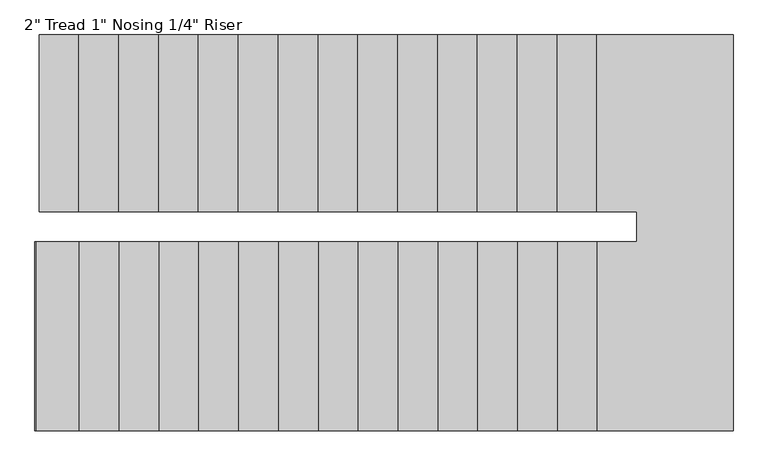
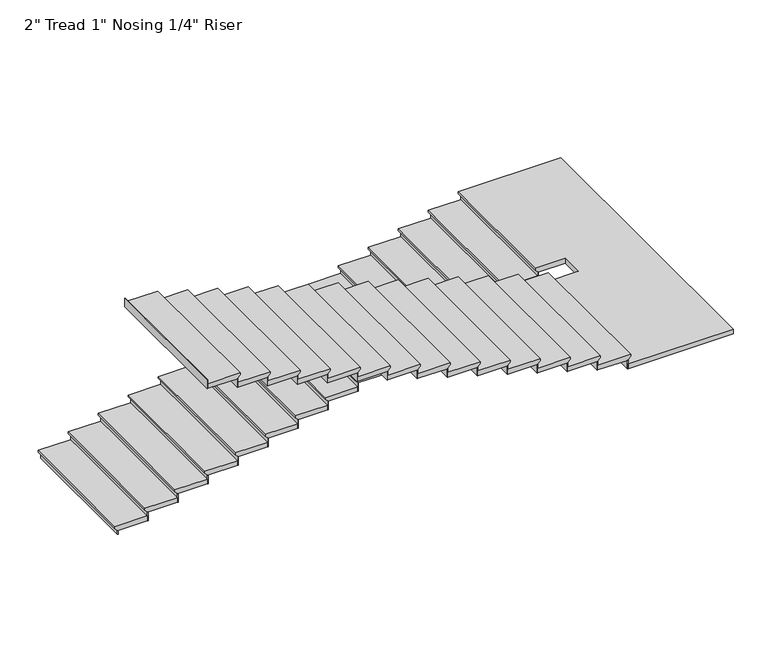
"""IFC4 building model written with IfcOpenShell, lengths in millimetres: stair flight geometry."""

from ifc_helpers import new_model, si_unit, origin, place, context, project, spatial, faceted_brep, source, transform, mapped, element, save


def stair_flight_0dc38caa(model_context):
    return source(origin(), model_context, "Body", "Brep", [
        faceted_brep([(-5254.0891351, 11154.2082924, 12264.39), (-5254.0891351, 11154.2082924, 12283.44), (-5254.0891351, 12506.0715905, 12283.44), (-5254.0891351, 12506.0715905, 12264.39), (-5228.6891351, 11154.2082924, 12238.99), (-5228.6891351, 12506.0715905, 12238.99), (-4923.8891351, 11154.2082924, 12283.44), (-4923.8891351, 12506.0715905, 12283.44), (-5228.6891351, 12506.0715905, 12232.64), (-4923.8891351, 12506.0715905, 12232.64), (-4923.8891351, 11154.2082924, 12232.64), (-5228.6891351, 11154.2082924, 12232.64)], [[[0, 1, 2, 3]], [[4, 0, 3, 5]], [[2, 1, 6, 7]], [[8, 9, 10, 11]], [[2, 7, 9, 8, 5, 3]], [[8, 11, 4, 5]], [[6, 1, 0, 4, 11, 10]], [[7, 6, 10, 9]]]),
        faceted_brep([(-5228.6891351, 11154.2082924, 12232.64), (-5228.6891351, 11154.2082924, 12192.0), (-5222.3391351, 11154.2082924, 12192.0), (-5222.3391351, 11154.2082924, 12232.64), (-5228.6891351, 12506.0715905, 12232.64), (-5222.3391351, 12506.0715905, 12232.64), (-5222.3391351, 12506.0715905, 12192.0), (-5228.6891351, 12506.0715905, 12192.0)], [[[0, 1, 2, 3]], [[4, 5, 6, 7]], [[1, 0, 4, 7]], [[2, 1, 7, 6]], [[3, 2, 6, 5]], [[0, 3, 5, 4]]]),
        faceted_brep([(-4923.8891351, 11154.2082924, 12324.08), (-4923.8891351, 11154.2082924, 12232.64), (-4917.5391351, 11154.2082924, 12232.64), (-4917.5391351, 11154.2082924, 12324.08), (-4923.8891351, 12506.0715905, 12324.08), (-4917.5391351, 12506.0715905, 12324.08), (-4917.5391351, 12506.0715905, 12232.64), (-4923.8891351, 12506.0715905, 12232.64)], [[[0, 1, 2, 3]], [[4, 5, 6, 7]], [[1, 0, 4, 7]], [[2, 1, 7, 6]], [[3, 2, 6, 5]], [[0, 3, 5, 4]]]),
        faceted_brep([(-4949.2891351, 12506.0715905, 12374.88), (-4949.2891351, 11154.2082924, 12374.88), (-4619.0891351, 11154.2082924, 12374.88), (-4619.0891351, 12506.0715905, 12374.88), (-4923.8891351, 12506.0715905, 12324.08), (-4619.0891351, 12506.0715905, 12324.08), (-4619.0891351, 11154.2082924, 12324.08), (-4923.8891351, 11154.2082924, 12324.08), (-4923.8891351, 12506.0715905, 12330.43), (-4949.2891351, 12506.0715905, 12355.83), (-4923.8891351, 11154.2082924, 12330.43), (-4949.2891351, 11154.2082924, 12355.83)], [[[0, 1, 2, 3]], [[4, 5, 6, 7]], [[0, 3, 5, 4, 8, 9]], [[4, 7, 10, 8]], [[2, 1, 11, 10, 7, 6]], [[3, 2, 6, 5]], [[11, 1, 0, 9]], [[10, 11, 9, 8]]]),
        faceted_brep([(-4619.0891351, 11154.2082924, 12415.52), (-4619.0891351, 11154.2082924, 12324.08), (-4612.7391351, 11154.2082924, 12324.08), (-4612.7391351, 11154.2082924, 12415.52), (-4619.0891351, 12506.0715905, 12415.52), (-4612.7391351, 12506.0715905, 12415.52), (-4612.7391351, 12506.0715905, 12324.08), (-4619.0891351, 12506.0715905, 12324.08)], [[[0, 1, 2, 3]], [[4, 5, 6, 7]], [[1, 0, 4, 7]], [[2, 1, 7, 6]], [[3, 2, 6, 5]], [[0, 3, 5, 4]]]),
        faceted_brep([(-4644.4891351, 12506.0715905, 12466.32), (-4644.4891351, 11154.2082924, 12466.32), (-4314.2891351, 11154.2082924, 12466.32), (-4314.2891351, 12506.0715905, 12466.32), (-4619.0891351, 12506.0715905, 12415.52), (-4314.2891351, 12506.0715905, 12415.52), (-4314.2891351, 11154.2082924, 12415.52), (-4619.0891351, 11154.2082924, 12415.52), (-4619.0891351, 12506.0715905, 12421.87), (-4644.4891351, 12506.0715905, 12447.27), (-4619.0891351, 11154.2082924, 12421.87), (-4644.4891351, 11154.2082924, 12447.27)], [[[0, 1, 2, 3]], [[4, 5, 6, 7]], [[0, 3, 5, 4, 8, 9]], [[4, 7, 10, 8]], [[2, 1, 11, 10, 7, 6]], [[3, 2, 6, 5]], [[11, 1, 0, 9]], [[10, 11, 9, 8]]]),
        faceted_brep([(-4314.2891351, 11154.2082924, 12506.96), (-4314.2891351, 11154.2082924, 12415.52), (-4307.9391351, 11154.2082924, 12415.52), (-4307.9391351, 11154.2082924, 12506.96), (-4314.2891351, 12506.0715905, 12506.96), (-4307.9391351, 12506.0715905, 12506.96), (-4307.9391351, 12506.0715905, 12415.52), (-4314.2891351, 12506.0715905, 12415.52)], [[[0, 1, 2, 3]], [[4, 5, 6, 7]], [[1, 0, 4, 7]], [[2, 1, 7, 6]], [[3, 2, 6, 5]], [[0, 3, 5, 4]]]),
        faceted_brep([(-4339.6891351, 12506.0715905, 12557.76), (-4339.6891351, 11154.2082924, 12557.76), (-4009.4891351, 11154.2082924, 12557.76), (-4009.4891351, 12506.0715905, 12557.76), (-4314.2891351, 12506.0715905, 12506.96), (-4009.4891351, 12506.0715905, 12506.96), (-4009.4891351, 11154.2082924, 12506.96), (-4314.2891351, 11154.2082924, 12506.96), (-4314.2891351, 12506.0715905, 12513.31), (-4339.6891351, 12506.0715905, 12538.71), (-4314.2891351, 11154.2082924, 12513.31), (-4339.6891351, 11154.2082924, 12538.71)], [[[0, 1, 2, 3]], [[4, 5, 6, 7]], [[0, 3, 5, 4, 8, 9]], [[4, 7, 10, 8]], [[2, 1, 11, 10, 7, 6]], [[3, 2, 6, 5]], [[11, 1, 0, 9]], [[10, 11, 9, 8]]]),
        faceted_brep([(-4009.4891351, 11154.2082924, 12598.4), (-4009.4891351, 11154.2082924, 12506.96), (-4003.1391351, 11154.2082924, 12506.96), (-4003.1391351, 11154.2082924, 12598.4), (-4009.4891351, 12506.0715905, 12598.4), (-4003.1391351, 12506.0715905, 12598.4), (-4003.1391351, 12506.0715905, 12506.96), (-4009.4891351, 12506.0715905, 12506.96)], [[[0, 1, 2, 3]], [[4, 5, 6, 7]], [[1, 0, 4, 7]], [[2, 1, 7, 6]], [[3, 2, 6, 5]], [[0, 3, 5, 4]]]),
        faceted_brep([(-4034.8891351, 12506.0715905, 12649.2), (-4034.8891351, 11154.2082924, 12649.2), (-3704.6891351, 11154.2082924, 12649.2), (-3704.6891351, 12506.0715905, 12649.2), (-4009.4891351, 12506.0715905, 12598.4), (-3704.6891351, 12506.0715905, 12598.4), (-3704.6891351, 11154.2082924, 12598.4), (-4009.4891351, 11154.2082924, 12598.4), (-4009.4891351, 12506.0715905, 12604.75), (-4034.8891351, 12506.0715905, 12630.15), (-4009.4891351, 11154.2082924, 12604.75), (-4034.8891351, 11154.2082924, 12630.15)], [[[0, 1, 2, 3]], [[4, 5, 6, 7]], [[0, 3, 5, 4, 8, 9]], [[4, 7, 10, 8]], [[2, 1, 11, 10, 7, 6]], [[3, 2, 6, 5]], [[11, 1, 0, 9]], [[10, 11, 9, 8]]]),
        faceted_brep([(-3704.6891351, 11154.2082924, 12689.84), (-3704.6891351, 11154.2082924, 12598.4), (-3698.3391351, 11154.2082924, 12598.4), (-3698.3391351, 11154.2082924, 12689.84), (-3704.6891351, 12506.0715905, 12689.84), (-3698.3391351, 12506.0715905, 12689.84), (-3698.3391351, 12506.0715905, 12598.4), (-3704.6891351, 12506.0715905, 12598.4)], [[[0, 1, 2, 3]], [[4, 5, 6, 7]], [[1, 0, 4, 7]], [[2, 1, 7, 6]], [[3, 2, 6, 5]], [[0, 3, 5, 4]]]),
        faceted_brep([(-3730.0891351, 12506.0715905, 12740.64), (-3730.0891351, 11154.2082924, 12740.64), (-3399.8891351, 11154.2082924, 12740.64), (-3399.8891351, 12506.0715905, 12740.64), (-3704.6891351, 12506.0715905, 12689.84), (-3399.8891351, 12506.0715905, 12689.84), (-3399.8891351, 11154.2082924, 12689.84), (-3704.6891351, 11154.2082924, 12689.84), (-3704.6891351, 12506.0715905, 12696.19), (-3730.0891351, 12506.0715905, 12721.59), (-3704.6891351, 11154.2082924, 12696.19), (-3730.0891351, 11154.2082924, 12721.59)], [[[0, 1, 2, 3]], [[4, 5, 6, 7]], [[0, 3, 5, 4, 8, 9]], [[4, 7, 10, 8]], [[2, 1, 11, 10, 7, 6]], [[3, 2, 6, 5]], [[11, 1, 0, 9]], [[10, 11, 9, 8]]]),
        faceted_brep([(-3399.8891351, 11154.2082924, 12781.28), (-3399.8891351, 11154.2082924, 12689.84), (-3393.5391351, 11154.2082924, 12689.84), (-3393.5391351, 11154.2082924, 12781.28), (-3399.8891351, 12506.0715905, 12781.28), (-3393.5391351, 12506.0715905, 12781.28), (-3393.5391351, 12506.0715905, 12689.84), (-3399.8891351, 12506.0715905, 12689.84)], [[[0, 1, 2, 3]], [[4, 5, 6, 7]], [[1, 0, 4, 7]], [[2, 1, 7, 6]], [[3, 2, 6, 5]], [[0, 3, 5, 4]]]),
        faceted_brep([(-3425.2891351, 12506.0715905, 12832.08), (-3425.2891351, 11154.2082924, 12832.08), (-3095.0891351, 11154.2082924, 12832.08), (-3095.0891351, 12506.0715905, 12832.08), (-3399.8891351, 12506.0715905, 12781.28), (-3095.0891351, 12506.0715905, 12781.28), (-3095.0891351, 11154.2082924, 12781.28), (-3399.8891351, 11154.2082924, 12781.28), (-3399.8891351, 12506.0715905, 12787.63), (-3425.2891351, 12506.0715905, 12813.03), (-3399.8891351, 11154.2082924, 12787.63), (-3425.2891351, 11154.2082924, 12813.03)], [[[0, 1, 2, 3]], [[4, 5, 6, 7]], [[0, 3, 5, 4, 8, 9]], [[4, 7, 10, 8]], [[2, 1, 11, 10, 7, 6]], [[3, 2, 6, 5]], [[11, 1, 0, 9]], [[10, 11, 9, 8]]]),
        faceted_brep([(-3095.0891351, 11154.2082924, 12872.72), (-3095.0891351, 11154.2082924, 12781.28), (-3088.7391351, 11154.2082924, 12781.28), (-3088.7391351, 11154.2082924, 12872.72), (-3095.0891351, 12506.0715905, 12872.72), (-3088.7391351, 12506.0715905, 12872.72), (-3088.7391351, 12506.0715905, 12781.28), (-3095.0891351, 12506.0715905, 12781.28)], [[[0, 1, 2, 3]], [[4, 5, 6, 7]], [[1, 0, 4, 7]], [[2, 1, 7, 6]], [[3, 2, 6, 5]], [[0, 3, 5, 4]]]),
        faceted_brep([(-3120.4891351, 12506.0715905, 12923.52), (-3120.4891351, 11154.2082924, 12923.52), (-2790.2891351, 11154.2082924, 12923.52), (-2790.2891351, 12506.0715905, 12923.52), (-3095.0891351, 12506.0715905, 12872.72), (-2790.2891351, 12506.0715905, 12872.72), (-2790.2891351, 11154.2082924, 12872.72), (-3095.0891351, 11154.2082924, 12872.72), (-3095.0891351, 12506.0715905, 12879.07), (-3120.4891351, 12506.0715905, 12904.47), (-3095.0891351, 11154.2082924, 12879.07), (-3120.4891351, 11154.2082924, 12904.47)], [[[0, 1, 2, 3]], [[4, 5, 6, 7]], [[0, 3, 5, 4, 8, 9]], [[4, 7, 10, 8]], [[2, 1, 11, 10, 7, 6]], [[3, 2, 6, 5]], [[11, 1, 0, 9]], [[10, 11, 9, 8]]]),
        faceted_brep([(-2790.2891351, 11154.2082924, 12964.16), (-2790.2891351, 11154.2082924, 12872.72), (-2783.9391351, 11154.2082924, 12872.72), (-2783.9391351, 11154.2082924, 12964.16), (-2790.2891351, 12506.0715905, 12964.16), (-2783.9391351, 12506.0715905, 12964.16), (-2783.9391351, 12506.0715905, 12872.72), (-2790.2891351, 12506.0715905, 12872.72)], [[[0, 1, 2, 3]], [[4, 5, 6, 7]], [[1, 0, 4, 7]], [[2, 1, 7, 6]], [[3, 2, 6, 5]], [[0, 3, 5, 4]]]),
        faceted_brep([(-2815.6891351, 12506.0715905, 13014.96), (-2815.6891351, 11154.2082924, 13014.96), (-2485.4891351, 11154.2082924, 13014.96), (-2485.4891351, 12506.0715905, 13014.96), (-2790.2891351, 12506.0715905, 12964.16), (-2485.4891351, 12506.0715905, 12964.16), (-2485.4891351, 11154.2082924, 12964.16), (-2790.2891351, 11154.2082924, 12964.16), (-2790.2891351, 12506.0715905, 12970.51), (-2815.6891351, 12506.0715905, 12995.91), (-2790.2891351, 11154.2082924, 12970.51), (-2815.6891351, 11154.2082924, 12995.91)], [[[0, 1, 2, 3]], [[4, 5, 6, 7]], [[0, 3, 5, 4, 8, 9]], [[4, 7, 10, 8]], [[2, 1, 11, 10, 7, 6]], [[3, 2, 6, 5]], [[11, 1, 0, 9]], [[10, 11, 9, 8]]]),
        faceted_brep([(-2485.4891351, 11154.2082924, 13055.6), (-2485.4891351, 11154.2082924, 12964.16), (-2479.1391351, 11154.2082924, 12964.16), (-2479.1391351, 11154.2082924, 13055.6), (-2485.4891351, 12506.0715905, 13055.6), (-2479.1391351, 12506.0715905, 13055.6), (-2479.1391351, 12506.0715905, 12964.16), (-2485.4891351, 12506.0715905, 12964.16)], [[[0, 1, 2, 3]], [[4, 5, 6, 7]], [[1, 0, 4, 7]], [[2, 1, 7, 6]], [[3, 2, 6, 5]], [[0, 3, 5, 4]]]),
        faceted_brep([(-2510.8891351, 12506.0715905, 13106.4), (-2510.8891351, 11154.2082924, 13106.4), (-2180.6891351, 11154.2082924, 13106.4), (-2180.6891351, 12506.0715905, 13106.4), (-2485.4891351, 12506.0715905, 13055.6), (-2180.6891351, 12506.0715905, 13055.6), (-2180.6891351, 11154.2082924, 13055.6), (-2485.4891351, 11154.2082924, 13055.6), (-2485.4891351, 12506.0715905, 13061.95), (-2510.8891351, 12506.0715905, 13087.35), (-2485.4891351, 11154.2082924, 13061.95), (-2510.8891351, 11154.2082924, 13087.35)], [[[0, 1, 2, 3]], [[4, 5, 6, 7]], [[0, 3, 5, 4, 8, 9]], [[4, 7, 10, 8]], [[2, 1, 11, 10, 7, 6]], [[3, 2, 6, 5]], [[11, 1, 0, 9]], [[10, 11, 9, 8]]]),
        faceted_brep([(-2180.6891351, 11154.2082924, 13147.04), (-2180.6891351, 11154.2082924, 13055.6), (-2174.3391351, 11154.2082924, 13055.6), (-2174.3391351, 11154.2082924, 13147.04), (-2180.6891351, 12506.0715905, 13147.04), (-2174.3391351, 12506.0715905, 13147.04), (-2174.3391351, 12506.0715905, 13055.6), (-2180.6891351, 12506.0715905, 13055.6)], [[[0, 1, 2, 3]], [[4, 5, 6, 7]], [[1, 0, 4, 7]], [[2, 1, 7, 6]], [[3, 2, 6, 5]], [[0, 3, 5, 4]]]),
        faceted_brep([(-2206.0891351, 12506.0715905, 13197.84), (-2206.0891351, 11154.2082924, 13197.84), (-1875.8891351, 11154.2082924, 13197.84), (-1875.8891351, 12506.0715905, 13197.84), (-2180.6891351, 12506.0715905, 13147.04), (-1875.8891351, 12506.0715905, 13147.04), (-1875.8891351, 11154.2082924, 13147.04), (-2180.6891351, 11154.2082924, 13147.04), (-2180.6891351, 12506.0715905, 13153.39), (-2206.0891351, 12506.0715905, 13178.79), (-2180.6891351, 11154.2082924, 13153.39), (-2206.0891351, 11154.2082924, 13178.79)], [[[0, 1, 2, 3]], [[4, 5, 6, 7]], [[0, 3, 5, 4, 8, 9]], [[4, 7, 10, 8]], [[2, 1, 11, 10, 7, 6]], [[3, 2, 6, 5]], [[11, 1, 0, 9]], [[10, 11, 9, 8]]]),
        faceted_brep([(-1875.8891351, 11154.2082924, 13238.48), (-1875.8891351, 11154.2082924, 13147.04), (-1869.5391351, 11154.2082924, 13147.04), (-1869.5391351, 11154.2082924, 13238.48), (-1875.8891351, 12506.0715905, 13238.48), (-1869.5391351, 12506.0715905, 13238.48), (-1869.5391351, 12506.0715905, 13147.04), (-1875.8891351, 12506.0715905, 13147.04)], [[[0, 1, 2, 3]], [[4, 5, 6, 7]], [[1, 0, 4, 7]], [[2, 1, 7, 6]], [[3, 2, 6, 5]], [[0, 3, 5, 4]]]),
        faceted_brep([(-1901.2891351, 12506.0715905, 13289.28), (-1901.2891351, 11154.2082924, 13289.28), (-1571.0891351, 11154.2082924, 13289.28), (-1571.0891351, 12506.0715905, 13289.28), (-1875.8891351, 12506.0715905, 13238.48), (-1571.0891351, 12506.0715905, 13238.48), (-1571.0891351, 11154.2082924, 13238.48), (-1875.8891351, 11154.2082924, 13238.48), (-1875.8891351, 12506.0715905, 13244.83), (-1901.2891351, 12506.0715905, 13270.23), (-1875.8891351, 11154.2082924, 13244.83), (-1901.2891351, 11154.2082924, 13270.23)], [[[0, 1, 2, 3]], [[4, 5, 6, 7]], [[0, 3, 5, 4, 8, 9]], [[4, 7, 10, 8]], [[2, 1, 11, 10, 7, 6]], [[3, 2, 6, 5]], [[11, 1, 0, 9]], [[10, 11, 9, 8]]]),
        faceted_brep([(-1571.0891351, 11154.2082924, 13329.92), (-1571.0891351, 11154.2082924, 13238.48), (-1564.7391351, 11154.2082924, 13238.48), (-1564.7391351, 11154.2082924, 13329.92), (-1571.0891351, 12506.0715905, 13329.92), (-1564.7391351, 12506.0715905, 13329.92), (-1564.7391351, 12506.0715905, 13238.48), (-1571.0891351, 12506.0715905, 13238.48)], [[[0, 1, 2, 3]], [[4, 5, 6, 7]], [[1, 0, 4, 7]], [[2, 1, 7, 6]], [[3, 2, 6, 5]], [[0, 3, 5, 4]]]),
        faceted_brep([(-1596.4891351, 12506.0715905, 13380.72), (-1596.4891351, 11154.2082924, 13380.72), (-1266.2891351, 11154.2082924, 13380.72), (-1266.2891351, 12506.0715905, 13380.72), (-1571.0891351, 12506.0715905, 13329.92), (-1266.2891351, 12506.0715905, 13329.92), (-1266.2891351, 11154.2082924, 13329.92), (-1571.0891351, 11154.2082924, 13329.92), (-1571.0891351, 12506.0715905, 13336.27), (-1596.4891351, 12506.0715905, 13361.67), (-1571.0891351, 11154.2082924, 13336.27), (-1596.4891351, 11154.2082924, 13361.67)], [[[0, 1, 2, 3]], [[4, 5, 6, 7]], [[0, 3, 5, 4, 8, 9]], [[4, 7, 10, 8]], [[2, 1, 11, 10, 7, 6]], [[3, 2, 6, 5]], [[11, 1, 0, 9]], [[10, 11, 9, 8]]]),
        faceted_brep([(-1266.2891351, 11154.2082924, 13421.36), (-1266.2891351, 11154.2082924, 13329.92), (-1259.9391351, 11154.2082924, 13329.92), (-1259.9391351, 11154.2082924, 13421.36), (-1266.2891351, 12506.0715905, 13421.36), (-1259.9391351, 12506.0715905, 13421.36), (-1259.9391351, 12506.0715905, 13329.92), (-1266.2891351, 12506.0715905, 13329.92)], [[[0, 1, 2, 3]], [[4, 5, 6, 7]], [[1, 0, 4, 7]], [[2, 1, 7, 6]], [[3, 2, 6, 5]], [[0, 3, 5, 4]]]),
        faceted_brep([(-1291.6891351, 12506.0715905, 13472.16), (-1291.6891351, 11154.2082924, 13472.16), (-961.4891351, 11154.2082924, 13472.16), (-961.4891351, 12506.0715905, 13472.16), (-1266.2891351, 12506.0715905, 13421.36), (-961.4891351, 12506.0715905, 13421.36), (-961.4891351, 11154.2082924, 13421.36), (-1266.2891351, 11154.2082924, 13421.36), (-1266.2891351, 12506.0715905, 13427.71), (-1291.6891351, 12506.0715905, 13453.11), (-1266.2891351, 11154.2082924, 13427.71), (-1291.6891351, 11154.2082924, 13453.11)], [[[0, 1, 2, 3]], [[4, 5, 6, 7]], [[0, 3, 5, 4, 8, 9]], [[4, 7, 10, 8]], [[2, 1, 11, 10, 7, 6]], [[3, 2, 6, 5]], [[11, 1, 0, 9]], [[10, 11, 9, 8]]]),
        faceted_brep([(-961.4891351, 11154.2082924, 13512.8), (-961.4891351, 11154.2082924, 13421.36), (-955.1391351, 11154.2082924, 13421.36), (-955.1391351, 11154.2082924, 13512.8), (-961.4891351, 12506.0715905, 13512.8), (-955.1391351, 12506.0715905, 13512.8), (-955.1391351, 12506.0715905, 13421.36), (-961.4891351, 12506.0715905, 13421.36)], [[[0, 1, 2, 3]], [[4, 5, 6, 7]], [[1, 0, 4, 7]], [[2, 1, 7, 6]], [[3, 2, 6, 5]], [[0, 3, 5, 4]]]),
        faceted_brep([(-1012.2891351, 9478.4949943, 13563.6), (54.5108649, 9478.4949943, 13563.6), (54.5108649, 12506.0715905, 13563.6), (-986.8891351, 12506.0715905, 13563.6), (-986.8891351, 11154.2082924, 13563.6), (-682.0891351, 11154.2082924, 13563.6), (-682.0891351, 10925.6082924, 13563.6), (-1012.2891351, 10925.6082924, 13563.6), (54.5108649, 9478.4949943, 13512.8), (-1012.2891351, 9478.4949943, 13512.8), (-1012.2891351, 10925.6082924, 13512.8), (-682.0891351, 10925.6082924, 13512.8), (-682.0891351, 11154.2082924, 13512.8), (-961.4891351, 11154.2082924, 13512.8), (-961.4891351, 12506.0715905, 13512.8), (54.5108649, 12506.0715905, 13512.8), (-961.4891351, 12506.0715905, 13519.15), (-986.8891351, 12506.0715905, 13544.55), (-961.4891351, 11154.2082924, 13519.15), (-986.8891351, 11154.2082924, 13544.55)], [[[0, 1, 2, 3, 4, 5, 6, 7]], [[8, 9, 10, 11, 12, 13, 14, 15]], [[1, 0, 9, 8]], [[2, 1, 8, 15]], [[3, 2, 15, 14, 16, 17]], [[14, 13, 18, 16]], [[5, 4, 19, 18, 13, 12]], [[6, 5, 12, 11]], [[7, 6, 11, 10]], [[0, 7, 10, 9]], [[19, 4, 3, 17]], [[18, 19, 17, 16]]]),
        faceted_brep([(-1012.2891351, 10925.6082924, 13604.24), (-1012.2891351, 10925.6082924, 13512.8), (-1018.6391351, 10925.6082924, 13512.8), (-1018.6391351, 10925.6082924, 13604.24), (-1012.2891351, 9478.4949943, 13604.24), (-1018.6391351, 9478.4949943, 13604.24), (-1018.6391351, 9478.4949943, 13512.8), (-1012.2891351, 9478.4949943, 13512.8)], [[[0, 1, 2, 3]], [[4, 5, 6, 7]], [[1, 0, 4, 7]], [[2, 1, 7, 6]], [[3, 2, 6, 5]], [[0, 3, 5, 4]]]),
        faceted_brep([(-986.8891351, 9478.4949943, 13655.04), (-986.8891351, 10925.6082924, 13655.04), (-1317.0891351, 10925.6082924, 13655.04), (-1317.0891351, 9478.4949943, 13655.04), (-1012.2891351, 9478.4949943, 13604.24), (-1317.0891351, 9478.4949943, 13604.24), (-1317.0891351, 10925.6082924, 13604.24), (-1012.2891351, 10925.6082924, 13604.24), (-1012.2891351, 9478.4949943, 13610.59), (-986.8891351, 9478.4949943, 13635.99), (-1012.2891351, 10925.6082924, 13610.59), (-986.8891351, 10925.6082924, 13635.99)], [[[0, 1, 2, 3]], [[4, 5, 6, 7]], [[0, 3, 5, 4, 8, 9]], [[4, 7, 10, 8]], [[2, 1, 11, 10, 7, 6]], [[3, 2, 6, 5]], [[11, 1, 0, 9]], [[10, 11, 9, 8]]]),
        faceted_brep([(-1317.0891351, 10925.6082924, 13695.68), (-1317.0891351, 10925.6082924, 13604.24), (-1323.4391351, 10925.6082924, 13604.24), (-1323.4391351, 10925.6082924, 13695.68), (-1317.0891351, 9478.4949943, 13695.68), (-1323.4391351, 9478.4949943, 13695.68), (-1323.4391351, 9478.4949943, 13604.24), (-1317.0891351, 9478.4949943, 13604.24)], [[[0, 1, 2, 3]], [[4, 5, 6, 7]], [[1, 0, 4, 7]], [[2, 1, 7, 6]], [[3, 2, 6, 5]], [[0, 3, 5, 4]]]),
        faceted_brep([(-1291.6891351, 9478.4949943, 13746.48), (-1291.6891351, 10925.6082924, 13746.48), (-1621.8891351, 10925.6082924, 13746.48), (-1621.8891351, 9478.4949943, 13746.48), (-1317.0891351, 9478.4949943, 13695.68), (-1621.8891351, 9478.4949943, 13695.68), (-1621.8891351, 10925.6082924, 13695.68), (-1317.0891351, 10925.6082924, 13695.68), (-1317.0891351, 9478.4949943, 13702.03), (-1291.6891351, 9478.4949943, 13727.43), (-1317.0891351, 10925.6082924, 13702.03), (-1291.6891351, 10925.6082924, 13727.43)], [[[0, 1, 2, 3]], [[4, 5, 6, 7]], [[0, 3, 5, 4, 8, 9]], [[4, 7, 10, 8]], [[2, 1, 11, 10, 7, 6]], [[3, 2, 6, 5]], [[11, 1, 0, 9]], [[10, 11, 9, 8]]]),
        faceted_brep([(-1621.8891351, 10925.6082924, 13787.12), (-1621.8891351, 10925.6082924, 13695.68), (-1628.2391351, 10925.6082924, 13695.68), (-1628.2391351, 10925.6082924, 13787.12), (-1621.8891351, 9478.4949943, 13787.12), (-1628.2391351, 9478.4949943, 13787.12), (-1628.2391351, 9478.4949943, 13695.68), (-1621.8891351, 9478.4949943, 13695.68)], [[[0, 1, 2, 3]], [[4, 5, 6, 7]], [[1, 0, 4, 7]], [[2, 1, 7, 6]], [[3, 2, 6, 5]], [[0, 3, 5, 4]]]),
        faceted_brep([(-1596.4891351, 9478.4949943, 13837.92), (-1596.4891351, 10925.6082924, 13837.92), (-1926.6891351, 10925.6082924, 13837.92), (-1926.6891351, 9478.4949943, 13837.92), (-1621.8891351, 9478.4949943, 13787.12), (-1926.6891351, 9478.4949943, 13787.12), (-1926.6891351, 10925.6082924, 13787.12), (-1621.8891351, 10925.6082924, 13787.12), (-1621.8891351, 9478.4949943, 13793.47), (-1596.4891351, 9478.4949943, 13818.87), (-1621.8891351, 10925.6082924, 13793.47), (-1596.4891351, 10925.6082924, 13818.87)], [[[0, 1, 2, 3]], [[4, 5, 6, 7]], [[0, 3, 5, 4, 8, 9]], [[4, 7, 10, 8]], [[2, 1, 11, 10, 7, 6]], [[3, 2, 6, 5]], [[11, 1, 0, 9]], [[10, 11, 9, 8]]]),
        faceted_brep([(-1926.6891351, 10925.6082924, 13878.56), (-1926.6891351, 10925.6082924, 13787.12), (-1933.0391351, 10925.6082924, 13787.12), (-1933.0391351, 10925.6082924, 13878.56), (-1926.6891351, 9478.4949943, 13878.56), (-1933.0391351, 9478.4949943, 13878.56), (-1933.0391351, 9478.4949943, 13787.12), (-1926.6891351, 9478.4949943, 13787.12)], [[[0, 1, 2, 3]], [[4, 5, 6, 7]], [[1, 0, 4, 7]], [[2, 1, 7, 6]], [[3, 2, 6, 5]], [[0, 3, 5, 4]]]),
        faceted_brep([(-1901.2891351, 9478.4949943, 13929.36), (-1901.2891351, 10925.6082924, 13929.36), (-2231.4891351, 10925.6082924, 13929.36), (-2231.4891351, 9478.4949943, 13929.36), (-1926.6891351, 9478.4949943, 13878.56), (-2231.4891351, 9478.4949943, 13878.56), (-2231.4891351, 10925.6082924, 13878.56), (-1926.6891351, 10925.6082924, 13878.56), (-1926.6891351, 9478.4949943, 13884.91), (-1901.2891351, 9478.4949943, 13910.31), (-1926.6891351, 10925.6082924, 13884.91), (-1901.2891351, 10925.6082924, 13910.31)], [[[0, 1, 2, 3]], [[4, 5, 6, 7]], [[0, 3, 5, 4, 8, 9]], [[4, 7, 10, 8]], [[2, 1, 11, 10, 7, 6]], [[3, 2, 6, 5]], [[11, 1, 0, 9]], [[10, 11, 9, 8]]]),
        faceted_brep([(-2231.4891351, 10925.6082924, 13970.0), (-2231.4891351, 10925.6082924, 13878.56), (-2237.8391351, 10925.6082924, 13878.56), (-2237.8391351, 10925.6082924, 13970.0), (-2231.4891351, 9478.4949943, 13970.0), (-2237.8391351, 9478.4949943, 13970.0), (-2237.8391351, 9478.4949943, 13878.56), (-2231.4891351, 9478.4949943, 13878.56)], [[[0, 1, 2, 3]], [[4, 5, 6, 7]], [[1, 0, 4, 7]], [[2, 1, 7, 6]], [[3, 2, 6, 5]], [[0, 3, 5, 4]]]),
        faceted_brep([(-2206.0891351, 9478.4949943, 14020.8), (-2206.0891351, 10925.6082924, 14020.8), (-2536.2891351, 10925.6082924, 14020.8), (-2536.2891351, 9478.4949943, 14020.8), (-2231.4891351, 9478.4949943, 13970.0), (-2536.2891351, 9478.4949943, 13970.0), (-2536.2891351, 10925.6082924, 13970.0), (-2231.4891351, 10925.6082924, 13970.0), (-2231.4891351, 9478.4949943, 13976.35), (-2206.0891351, 9478.4949943, 14001.75), (-2231.4891351, 10925.6082924, 13976.35), (-2206.0891351, 10925.6082924, 14001.75)], [[[0, 1, 2, 3]], [[4, 5, 6, 7]], [[0, 3, 5, 4, 8, 9]], [[4, 7, 10, 8]], [[2, 1, 11, 10, 7, 6]], [[3, 2, 6, 5]], [[11, 1, 0, 9]], [[10, 11, 9, 8]]]),
        faceted_brep([(-2536.2891351, 10925.6082924, 14061.44), (-2536.2891351, 10925.6082924, 13970.0), (-2542.6391351, 10925.6082924, 13970.0), (-2542.6391351, 10925.6082924, 14061.44), (-2536.2891351, 9478.4949943, 14061.44), (-2542.6391351, 9478.4949943, 14061.44), (-2542.6391351, 9478.4949943, 13970.0), (-2536.2891351, 9478.4949943, 13970.0)], [[[0, 1, 2, 3]], [[4, 5, 6, 7]], [[1, 0, 4, 7]], [[2, 1, 7, 6]], [[3, 2, 6, 5]], [[0, 3, 5, 4]]]),
        faceted_brep([(-2510.8891351, 9478.4949943, 14112.24), (-2510.8891351, 10925.6082924, 14112.24), (-2841.0891351, 10925.6082924, 14112.24), (-2841.0891351, 9478.4949943, 14112.24), (-2536.2891351, 9478.4949943, 14061.44), (-2841.0891351, 9478.4949943, 14061.44), (-2841.0891351, 10925.6082924, 14061.44), (-2536.2891351, 10925.6082924, 14061.44), (-2536.2891351, 9478.4949943, 14067.79), (-2510.8891351, 9478.4949943, 14093.19), (-2536.2891351, 10925.6082924, 14067.79), (-2510.8891351, 10925.6082924, 14093.19)], [[[0, 1, 2, 3]], [[4, 5, 6, 7]], [[0, 3, 5, 4, 8, 9]], [[4, 7, 10, 8]], [[2, 1, 11, 10, 7, 6]], [[3, 2, 6, 5]], [[11, 1, 0, 9]], [[10, 11, 9, 8]]]),
        faceted_brep([(-2841.0891351, 10925.6082924, 14152.88), (-2841.0891351, 10925.6082924, 14061.44), (-2847.4391351, 10925.6082924, 14061.44), (-2847.4391351, 10925.6082924, 14152.88), (-2841.0891351, 9478.4949943, 14152.88), (-2847.4391351, 9478.4949943, 14152.88), (-2847.4391351, 9478.4949943, 14061.44), (-2841.0891351, 9478.4949943, 14061.44)], [[[0, 1, 2, 3]], [[4, 5, 6, 7]], [[1, 0, 4, 7]], [[2, 1, 7, 6]], [[3, 2, 6, 5]], [[0, 3, 5, 4]]]),
        faceted_brep([(-2815.6891351, 9478.4949943, 14203.68), (-2815.6891351, 10925.6082924, 14203.68), (-3145.8891351, 10925.6082924, 14203.68), (-3145.8891351, 9478.4949943, 14203.68), (-2841.0891351, 9478.4949943, 14152.88), (-3145.8891351, 9478.4949943, 14152.88), (-3145.8891351, 10925.6082924, 14152.88), (-2841.0891351, 10925.6082924, 14152.88), (-2841.0891351, 9478.4949943, 14159.23), (-2815.6891351, 9478.4949943, 14184.63), (-2841.0891351, 10925.6082924, 14159.23), (-2815.6891351, 10925.6082924, 14184.63)], [[[0, 1, 2, 3]], [[4, 5, 6, 7]], [[0, 3, 5, 4, 8, 9]], [[4, 7, 10, 8]], [[2, 1, 11, 10, 7, 6]], [[3, 2, 6, 5]], [[11, 1, 0, 9]], [[10, 11, 9, 8]]]),
        faceted_brep([(-3145.8891351, 10925.6082924, 14244.32), (-3145.8891351, 10925.6082924, 14152.88), (-3152.2391351, 10925.6082924, 14152.88), (-3152.2391351, 10925.6082924, 14244.32), (-3145.8891351, 9478.4949943, 14244.32), (-3152.2391351, 9478.4949943, 14244.32), (-3152.2391351, 9478.4949943, 14152.88), (-3145.8891351, 9478.4949943, 14152.88)], [[[0, 1, 2, 3]], [[4, 5, 6, 7]], [[1, 0, 4, 7]], [[2, 1, 7, 6]], [[3, 2, 6, 5]], [[0, 3, 5, 4]]]),
        faceted_brep([(-3120.4891351, 9478.4949943, 14295.12), (-3120.4891351, 10925.6082924, 14295.12), (-3450.6891351, 10925.6082924, 14295.12), (-3450.6891351, 9478.4949943, 14295.12), (-3145.8891351, 9478.4949943, 14244.32), (-3450.6891351, 9478.4949943, 14244.32), (-3450.6891351, 10925.6082924, 14244.32), (-3145.8891351, 10925.6082924, 14244.32), (-3145.8891351, 9478.4949943, 14250.67), (-3120.4891351, 9478.4949943, 14276.07), (-3145.8891351, 10925.6082924, 14250.67), (-3120.4891351, 10925.6082924, 14276.07)], [[[0, 1, 2, 3]], [[4, 5, 6, 7]], [[0, 3, 5, 4, 8, 9]], [[4, 7, 10, 8]], [[2, 1, 11, 10, 7, 6]], [[3, 2, 6, 5]], [[11, 1, 0, 9]], [[10, 11, 9, 8]]]),
        faceted_brep([(-3450.6891351, 10925.6082924, 14335.76), (-3450.6891351, 10925.6082924, 14244.32), (-3457.0391351, 10925.6082924, 14244.32), (-3457.0391351, 10925.6082924, 14335.76), (-3450.6891351, 9478.4949943, 14335.76), (-3457.0391351, 9478.4949943, 14335.76), (-3457.0391351, 9478.4949943, 14244.32), (-3450.6891351, 9478.4949943, 14244.32)], [[[0, 1, 2, 3]], [[4, 5, 6, 7]], [[1, 0, 4, 7]], [[2, 1, 7, 6]], [[3, 2, 6, 5]], [[0, 3, 5, 4]]]),
        faceted_brep([(-3425.2891351, 9478.4949943, 14386.56), (-3425.2891351, 10925.6082924, 14386.56), (-3755.4891351, 10925.6082924, 14386.56), (-3755.4891351, 9478.4949943, 14386.56), (-3450.6891351, 9478.4949943, 14335.76), (-3755.4891351, 9478.4949943, 14335.76), (-3755.4891351, 10925.6082924, 14335.76), (-3450.6891351, 10925.6082924, 14335.76), (-3450.6891351, 9478.4949943, 14342.11), (-3425.2891351, 9478.4949943, 14367.51), (-3450.6891351, 10925.6082924, 14342.11), (-3425.2891351, 10925.6082924, 14367.51)], [[[0, 1, 2, 3]], [[4, 5, 6, 7]], [[0, 3, 5, 4, 8, 9]], [[4, 7, 10, 8]], [[2, 1, 11, 10, 7, 6]], [[3, 2, 6, 5]], [[11, 1, 0, 9]], [[10, 11, 9, 8]]]),
        faceted_brep([(-3755.4891351, 10925.6082924, 14427.2), (-3755.4891351, 10925.6082924, 14335.76), (-3761.8391351, 10925.6082924, 14335.76), (-3761.8391351, 10925.6082924, 14427.2), (-3755.4891351, 9478.4949943, 14427.2), (-3761.8391351, 9478.4949943, 14427.2), (-3761.8391351, 9478.4949943, 14335.76), (-3755.4891351, 9478.4949943, 14335.76)], [[[0, 1, 2, 3]], [[4, 5, 6, 7]], [[1, 0, 4, 7]], [[2, 1, 7, 6]], [[3, 2, 6, 5]], [[0, 3, 5, 4]]]),
        faceted_brep([(-3730.0891351, 9478.4949943, 14478.0), (-3730.0891351, 10925.6082924, 14478.0), (-4060.2891351, 10925.6082924, 14478.0), (-4060.2891351, 9478.4949943, 14478.0), (-3755.4891351, 9478.4949943, 14427.2), (-4060.2891351, 9478.4949943, 14427.2), (-4060.2891351, 10925.6082924, 14427.2), (-3755.4891351, 10925.6082924, 14427.2), (-3755.4891351, 9478.4949943, 14433.55), (-3730.0891351, 9478.4949943, 14458.95), (-3755.4891351, 10925.6082924, 14433.55), (-3730.0891351, 10925.6082924, 14458.95)], [[[0, 1, 2, 3]], [[4, 5, 6, 7]], [[0, 3, 5, 4, 8, 9]], [[4, 7, 10, 8]], [[2, 1, 11, 10, 7, 6]], [[3, 2, 6, 5]], [[11, 1, 0, 9]], [[10, 11, 9, 8]]]),
        faceted_brep([(-4060.2891351, 10925.6082924, 14518.64), (-4060.2891351, 10925.6082924, 14427.2), (-4066.6391351, 10925.6082924, 14427.2), (-4066.6391351, 10925.6082924, 14518.64), (-4060.2891351, 9478.4949943, 14518.64), (-4066.6391351, 9478.4949943, 14518.64), (-4066.6391351, 9478.4949943, 14427.2), (-4060.2891351, 9478.4949943, 14427.2)], [[[0, 1, 2, 3]], [[4, 5, 6, 7]], [[1, 0, 4, 7]], [[2, 1, 7, 6]], [[3, 2, 6, 5]], [[0, 3, 5, 4]]]),
        faceted_brep([(-4034.8891351, 9478.4949943, 14569.44), (-4034.8891351, 10925.6082924, 14569.44), (-4365.0891351, 10925.6082924, 14569.44), (-4365.0891351, 9478.4949943, 14569.44), (-4060.2891351, 9478.4949943, 14518.64), (-4365.0891351, 9478.4949943, 14518.64), (-4365.0891351, 10925.6082924, 14518.64), (-4060.2891351, 10925.6082924, 14518.64), (-4060.2891351, 9478.4949943, 14524.99), (-4034.8891351, 9478.4949943, 14550.39), (-4060.2891351, 10925.6082924, 14524.99), (-4034.8891351, 10925.6082924, 14550.39)], [[[0, 1, 2, 3]], [[4, 5, 6, 7]], [[0, 3, 5, 4, 8, 9]], [[4, 7, 10, 8]], [[2, 1, 11, 10, 7, 6]], [[3, 2, 6, 5]], [[11, 1, 0, 9]], [[10, 11, 9, 8]]]),
        faceted_brep([(-4365.0891351, 10925.6082924, 14610.08), (-4365.0891351, 10925.6082924, 14518.64), (-4371.4391351, 10925.6082924, 14518.64), (-4371.4391351, 10925.6082924, 14610.08), (-4365.0891351, 9478.4949943, 14610.08), (-4371.4391351, 9478.4949943, 14610.08), (-4371.4391351, 9478.4949943, 14518.64), (-4365.0891351, 9478.4949943, 14518.64)], [[[0, 1, 2, 3]], [[4, 5, 6, 7]], [[1, 0, 4, 7]], [[2, 1, 7, 6]], [[3, 2, 6, 5]], [[0, 3, 5, 4]]]),
        faceted_brep([(-4339.6891351, 9478.4949943, 14660.88), (-4339.6891351, 10925.6082924, 14660.88), (-4669.8891351, 10925.6082924, 14660.88), (-4669.8891351, 9478.4949943, 14660.88), (-4365.0891351, 9478.4949943, 14610.08), (-4669.8891351, 9478.4949943, 14610.08), (-4669.8891351, 10925.6082924, 14610.08), (-4365.0891351, 10925.6082924, 14610.08), (-4365.0891351, 9478.4949943, 14616.43), (-4339.6891351, 9478.4949943, 14641.83), (-4365.0891351, 10925.6082924, 14616.43), (-4339.6891351, 10925.6082924, 14641.83)], [[[0, 1, 2, 3]], [[4, 5, 6, 7]], [[0, 3, 5, 4, 8, 9]], [[4, 7, 10, 8]], [[2, 1, 11, 10, 7, 6]], [[3, 2, 6, 5]], [[11, 1, 0, 9]], [[10, 11, 9, 8]]]),
        faceted_brep([(-4669.8891351, 10925.6082924, 14701.52), (-4669.8891351, 10925.6082924, 14610.08), (-4676.2391351, 10925.6082924, 14610.08), (-4676.2391351, 10925.6082924, 14701.52), (-4669.8891351, 9478.4949943, 14701.52), (-4676.2391351, 9478.4949943, 14701.52), (-4676.2391351, 9478.4949943, 14610.08), (-4669.8891351, 9478.4949943, 14610.08)], [[[0, 1, 2, 3]], [[4, 5, 6, 7]], [[1, 0, 4, 7]], [[2, 1, 7, 6]], [[3, 2, 6, 5]], [[0, 3, 5, 4]]]),
        faceted_brep([(-4644.4891351, 9478.4949943, 14752.32), (-4644.4891351, 10925.6082924, 14752.32), (-4974.6891351, 10925.6082924, 14752.32), (-4974.6891351, 9478.4949943, 14752.32), (-4669.8891351, 9478.4949943, 14701.52), (-4974.6891351, 9478.4949943, 14701.52), (-4974.6891351, 10925.6082924, 14701.52), (-4669.8891351, 10925.6082924, 14701.52), (-4669.8891351, 9478.4949943, 14707.87), (-4644.4891351, 9478.4949943, 14733.27), (-4669.8891351, 10925.6082924, 14707.87), (-4644.4891351, 10925.6082924, 14733.27)], [[[0, 1, 2, 3]], [[4, 5, 6, 7]], [[0, 3, 5, 4, 8, 9]], [[4, 7, 10, 8]], [[2, 1, 11, 10, 7, 6]], [[3, 2, 6, 5]], [[11, 1, 0, 9]], [[10, 11, 9, 8]]]),
        faceted_brep([(-4974.6891351, 10925.6082924, 14792.96), (-4974.6891351, 10925.6082924, 14701.52), (-4981.0391351, 10925.6082924, 14701.52), (-4981.0391351, 10925.6082924, 14792.96), (-4974.6891351, 9478.4949943, 14792.96), (-4981.0391351, 9478.4949943, 14792.96), (-4981.0391351, 9478.4949943, 14701.52), (-4974.6891351, 9478.4949943, 14701.52)], [[[0, 1, 2, 3]], [[4, 5, 6, 7]], [[1, 0, 4, 7]], [[2, 1, 7, 6]], [[3, 2, 6, 5]], [[0, 3, 5, 4]]]),
        faceted_brep([(-5279.4891351, 10925.6082924, 14884.4), (-5279.4891351, 10925.6082924, 14792.96), (-5285.8391351, 10925.6082924, 14792.96), (-5285.8391351, 10925.6082924, 14884.4), (-5279.4891351, 9478.4949943, 14884.4), (-5285.8391351, 9478.4949943, 14884.4), (-5285.8391351, 9478.4949943, 14792.96), (-5279.4891351, 9478.4949943, 14792.96)], [[[0, 1, 2, 3]], [[4, 5, 6, 7]], [[1, 0, 4, 7]], [[2, 1, 7, 6]], [[3, 2, 6, 5]], [[0, 3, 5, 4]]]),
        faceted_brep([(-4949.2891351, 9478.4949943, 14843.76), (-4949.2891351, 10925.6082924, 14843.76), (-5279.4891351, 10925.6082924, 14843.76), (-5279.4891351, 9478.4949943, 14843.76), (-4974.6891351, 9478.4949943, 14792.96), (-5279.4891351, 9478.4949943, 14792.96), (-5279.4891351, 10925.6082924, 14792.96), (-4974.6891351, 10925.6082924, 14792.96), (-4974.6891351, 9478.4949943, 14799.31), (-4949.2891351, 9478.4949943, 14824.71), (-4974.6891351, 10925.6082924, 14799.31), (-4949.2891351, 10925.6082924, 14824.71)], [[[0, 1, 2, 3]], [[4, 5, 6, 7]], [[0, 3, 5, 4, 8, 9]], [[4, 7, 10, 8]], [[2, 1, 11, 10, 7, 6]], [[3, 2, 6, 5]], [[11, 1, 0, 9]], [[10, 11, 9, 8]]]),
    ])


if __name__ == "__main__":
    model = new_model("IFC4")
    model_context = context("Model", 3, world=origin())
    ifc_project = project(units=[si_unit("LENGTHUNIT", "METRE", prefix="MILLI")], contexts=[model_context])
    site = spatial("IfcSite", under=ifc_project)
    building = spatial("IfcBuilding", under=site)
    placement = place(None, origin())
    stair_flight_shape = stair_flight_0dc38caa(model_context)
    element("IfcStairFlight", 1, ObjectType="2\" Tread 1\" Nosing 1/4\" Riser", at=placement, inside=building, context=model_context, shape_type="MappedRepresentation", body=[
        mapped(stair_flight_shape, transform((0.0, 0.0, 0.0), x_axis=(1.0, 0.0, 0.0), y_axis=(0.0, 1.0, 0.0), z_axis=(0.0, 0.0, 1.0))),
    ])
    save(model, "model.ifc")
